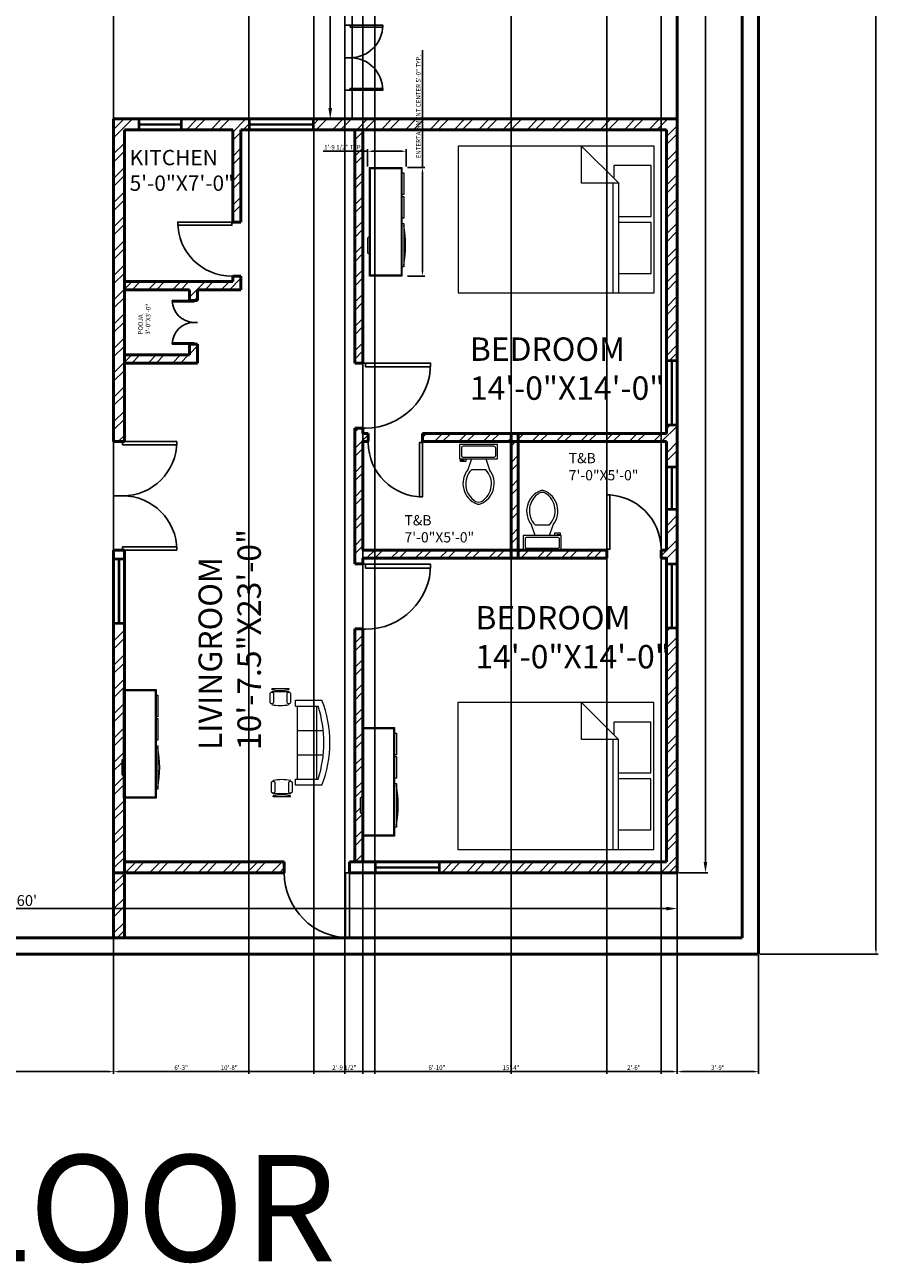
# Model space of a CAD drawing. Units: inches. Extents: x -12550 to 6516, y 1273 to 18700.
# Tile 3 of 19: x 2377 to 2849, y 1273 to 1958. Entities that reach past the tile are written whole.
import ezdxf

# ---------------------------------------------------------------- set-up
doc = ezdxf.new("R2010")
doc.units = ezdxf.units.IN
for name, color, linetype, lineweight in [('A-ANNO-DIMS', 2, 'Continuous', 18), ('A-ANNO-TEXT', 7, 'Continuous', 25), ('A-AREA-IDEN', 1, 'Continuous', 18), ('A-DOOR', 5, 'Continuous', 25), ('A-EQPM', 4, 'Continuous', 25), ('A-FURN', 8, 'Continuous', 18), ('A-GLAZ', 3, 'Continuous', 25), ('A-WALL', 7, 'Continuous', 50), ('A-WALL-PATT', 8, 'Continuous', 13)]:
    doc.layers.add(name, color=color, linetype=linetype, lineweight=lineweight)
doc.styles.get("Standard").update_dxf_attribs({"font": 'arial.ttf'})
doc.dimstyles.new('ISO-25', dxfattribs={"dimtxt": 2.5, "dimasz": 2.5, "dimexe": 1.25, "dimexo": 0.625, "dimtad": 1, "dimlunit": 4, "dimtxsty": 'Standard', "dimcen": 2.5, "dimadec": 0, "dimazin": 0, "dimtfac": 1, "dimtmove": 0, "dimatfit": 3, "dimfxl": 1, "dimarcsym": 0})

# ---------------------------------------------------------------- blocks, each defined once
blk = doc.blocks.new('*U2')
for p, q in [((0, 0), (0, -5)), ((30, 0), (30, -5))]:
    blk.add_line(p, q)
blk.add_lwpolyline([(0, 0), (0, 30), (1.75, 30), (1.75, 0)], close=True)
blk.add_arc((0, 0), 30, 0, 90)
blk = doc.blocks.new('Bed - Queen')
for p, q in [((0, -80.00003), (0, 0)), ((0, 0), (59.99999, 0)), ((59.99999, 0), (59.99999, -80.00003)), ((7.99999, -1.2), (28.79998, -1.2)), ((7.99999, -14.4), (7.99999, -1.2)), ((28.79998, -1.2), (28.79998, -14.4)), ((31.19999, -1.2), (51.99999, -1.2)), ((31.19999, -14.4), (31.19999, -1.2)), ((51.99999, -1.2), (51.99999, -16.4)), ((0, -14.4), (44.8, -14.4)), ((59.99999, -29.6), (44.8, -14.4)), ((44.8, -14.4), (44.8, -29.6)), ((44.8, -16.8), (0, -16.8)), ((51.99999, -16.4), (46.79936, -16.4)), ((44.8, -29.6), (59.99999, -29.6)), ((59.99999, -80.00003), (0, -80.00003))]:
    blk.add_line(p, q)
blk = doc.blocks.new('Toilet - top')
for p, q in [((9.5, -6), (9.5, -2)), ((-10, -8.5), (-8, -8.5)), ((-10, -9.5), (-10, -8.5)), ((-7, -9.5), (-10, -9.5)), ((-8, -8.5), (-8, -8)), ((-7, -8), (-7, -9.5)), ((-4, -8), (-6, -14)), ((4, -8), (6, -14)), ((4, -14), (-4, -14))]:
    blk.add_line(p, q)
blk.add_lwpolyline([(10.5, -8), (10.5, 0), (-10.5, 0), (-10.5, -8)], close=True)
for points in [[(-9.5, -2), (-9.5, -6)], [(8.5, -1), (-8.5, -1)], [(-8.5, -7), (8.5, -7)]]:
    blk.add_lwpolyline(points)
for centre, radius, start, end in [((-8.62, -1.88), 0.884, 81.8699, 188.1301), ((-8.62, -6.12), 0.884, 171.8699, 278.1301), ((8.62, -1.88), 0.884, 351.8699, 98.1301), ((8.62, -6.12), 0.884, 261.8699, 8.1301), ((3.52, -21.58), 12.17, 141.46911, 247.97143), ((4.2, -21.82), 11.33, 136.36773, 238.94682), ((-3.52, -21.58), 12.17, 292.02843, 38.53071), ((-4.2, -21.82), 11.33, 301.05301, 43.63209), ((0, -27.88), 4, 245.73182, 294.26817), ((0, -29), 4, 254.86053, 285.13947)]:
    blk.add_arc(centre, radius, start, end)
blk = doc.blocks.new('Entertainment Center')
for p, q in [((-4, 0), (-5, -1)), ((4, 0), (-4, 0)), ((5, -1), (4, 0)), ((-17, -19), (-17, -1)), ((-17, -1), (43, -1)), ((-16.5, -18.5), (-16.5, -1.5)), ((-16.5, -1.5), (42.5, -1.5)), ((42.5, -1.5), (42.5, -18.5)), ((43, -1), (43, -19)), ((43, -19), (-17, -19)), ((42.5, -18.5), (-16.5, -18.5)), ((-12, -20), (-12, -19)), ((12, -20), (-12, -20)), ((12, -19), (12, -20)), ((15, -20), (15, -19)), ((27, -20), (15, -20)), ((27, -19), (27, -20)), ((28, -20), (28, -19)), ((40, -20), (28, -20)), ((40, -19), (40, -20))]:
    blk.add_line(p, q)
blk.add_arc((0, 40), 61, 259.6111, 280.3889)
blk = doc.blocks.new('Sofa - Roundback 7 ft.')
for p, q in [((-36.000027, -34), (-36.000027, -11.4696)), ((-12.00002, -32.4421), (-12.00003, -6.5971)), ((11.99997, -32.4421), (11.99998, -6.5971)), ((35.99998, -34), (35.99998, -11.4696)), ((-35.999844, -13.3819), (35.9998, -13.3819)), ((-36.000027, -32.4421), (35.99998, -32.4421))]:
    blk.add_line(p, q)
for points in [[(-36.000027, -34), (-42.000027, -34), (-42.000027, -8)], [(41.99998, -8), (41.99998, -34), (35.99998, -34)]]:
    blk.add_lwpolyline(points)
for centre, radius, start, end in [((0, -114.25), 114.25, 68.43141, 111.5686), ((-0.00001, -127.1968), 121.1968, 72.72033, 107.2797)]:
    blk.add_arc(centre, radius, start, end)
blk = doc.blocks.new('Chair - Desk')
for p, q in [((-8.5, 0), (-8.5, -1)), ((-8.5, 0), (8.5, 0)), ((8.5, 0), (8.5, -1)), ((-10.5, -5), (-10.5, -14)), ((-8.5, -3), (-8.5, -4)), ((-8.5, -3), (8.5, -3)), ((-6.5, -14), (-6.5, -5)), ((-2, -3), (-2, -1.9355)), ((2, -1.9576), (2, -3)), ((6.5, -5), (6.5, -14)), ((8.5, -3), (8.5, -4)), ((10.5, -14), (10.5, -5)), ((-8.5, -15), (-8.5, -16)), ((8.5, -15), (8.5, -16))]:
    blk.add_line(p, q)
for centre, radius, start, end in [((-8.5, -6.5), 2.5, 36.8699, 143.1301), ((0, 34.625), 36.625, 256.5803, 283.4197), ((8.5, -6.5), 2.5, 36.8699, 143.1301), ((-8.5, -12.5), 2.5, 216.8699, 323.1301), ((0, 19.625), 36.625, 256.5803, 283.4197), ((8.5, -12.5), 2.5, 216.8699, 323.1301)]:
    blk.add_arc(centre, radius, start, end)
blk = doc.blocks.new('*D14')
at = {"layer": 'A-ANNO-DIMS', "color": 0, "lineweight": -2, "transparency": 16777216}
for p, q in [((2553.06, 2056.25), (2544.35, 2056.25)), ((2545.6, 2050.25), (2545.6, 1912.25)), ((2553.06, 1906.25), (2544.35, 1906.25))]:
    blk.add_line(p, q, dxfattribs=at)
at = {"layer": 'A-ANNO-DIMS', "color": 0, "transparency": 16777216}
for points in [[(2544.6, 2050.25), (2546.6, 2050.25), (2545.6, 2056.25)], [(2544.6, 1912.25), (2546.6, 1912.25), (2545.6, 1906.25)]]:
    blk.add_solid(points, dxfattribs=at)
at = {"layer": 'Defpoints', "color": 0, "transparency": 16777216}
for p in [(2553.69, 2056.25), (2545.6, 1906.25), (2553.69, 1906.25)]:
    blk.add_point(p, dxfattribs=at)
at = {"layer": 'A-ANNO-DIMS', "color": 0, "transparency": 16777216, "insert": (2541.91, 1981.25), "char_height": 6, "attachment_point": 5, "rotation": 90}
blk.add_mtext('12\'-6"', dxfattribs=at)
blk = doc.blocks.new('*D16')
at = {"layer": 'A-ANNO-DIMS', "color": 0, "lineweight": -2, "transparency": 16777216}
for p, q in [((2738.31, 2473.25), (2754.56, 2473.25)), ((2753.31, 2467.25), (2753.31, 1495.25)), ((2738.31, 1489.25), (2754.56, 1489.25))]:
    blk.add_line(p, q, dxfattribs=at)
at = {"layer": 'A-ANNO-DIMS', "color": 0, "transparency": 16777216}
for points in [[(2752.31, 2467.25), (2754.31, 2467.25), (2753.31, 2473.25)], [(2752.31, 1495.25), (2754.31, 1495.25), (2753.31, 1489.25)]]:
    blk.add_solid(points, dxfattribs=at)
at = {"layer": 'Defpoints', "color": 0, "transparency": 16777216}
for p in [(2737.69, 2473.25), (2737.69, 1489.25), (2753.31, 1489.25)]:
    blk.add_point(p, dxfattribs=at)
at = {"layer": 'A-ANNO-DIMS', "color": 0, "transparency": 16777216, "insert": (2749.62, 1981.25), "char_height": 6, "attachment_point": 5, "rotation": 90}
blk.add_mtext("82'", dxfattribs=at)
blk = doc.blocks.new('*D17')
at = {"layer": 'A-ANNO-DIMS', "color": 0, "lineweight": -2, "transparency": 16777216}
for p, q in [((2017.69, 1488.62), (2017.69, 1468.21)), ((2737.69, 1488.62), (2737.69, 1468.21)), ((2731.69, 1469.46), (2023.69, 1469.46))]:
    blk.add_line(p, q, dxfattribs=at)
at = {"layer": 'A-ANNO-DIMS', "color": 0, "transparency": 16777216}
for points in [[(2023.69, 1470.46), (2023.69, 1468.46), (2017.69, 1469.46)], [(2731.69, 1470.46), (2731.69, 1468.46), (2737.69, 1469.46)]]:
    blk.add_solid(points, dxfattribs=at)
at = {"layer": 'Defpoints', "color": 0, "transparency": 16777216}
for p in [(2017.69, 1489.25), (2737.69, 1489.25), (2017.69, 1469.46)]:
    blk.add_point(p, dxfattribs=at)
at = {"layer": 'A-ANNO-DIMS', "color": 0, "transparency": 16777216, "insert": (2377.69, 1473.15), "char_height": 6, "attachment_point": 5}
blk.add_mtext("60'", dxfattribs=at)
blk = doc.blocks.new('WIN-3FT')
for p, q in [((0, 0), (0, 6)), ((0, 6), (36.02, 6)), ((36.02, 0), (0, 0)), ((0.5, 0), (0.5, 6)), ((35.52, 3.2), (0.5, 3.2)), ((35.52, 2.8), (0.5, 2.8)), ((35.52, 6), (35.52, 0)), ((36.02, 6), (36.02, 0))]:
    blk.add_line(p, q)
blk = doc.blocks.new('WIN-2FT')
for p, q in [((0, 0), (0, 24.02)), ((0, 24.02), (6, 24.02)), ((0, 23.52), (6, 23.52)), ((2.8, 0.5), (2.8, 23.52)), ((3.2, 0.5), (3.2, 23.52)), ((6, 24.02), (6, 0)), ((6, 0.5), (0, 0.5)), ((6, 0), (0, 0))]:
    blk.add_line(p, q)
blk = doc.blocks.new('*D67')
at = {"layer": 'A-ANNO-DIMS', "color": 0, "lineweight": -2, "transparency": 16777216}
for p, q in [((2596.65, 1879.38), (2596.65, 1944.22)), ((2588.28, 1879.38), (2597.9, 1879.38)), ((2596.65, 1821.88), (2596.65, 1876.88)), ((2588.28, 1819.38), (2597.9, 1819.38))]:
    blk.add_line(p, q, dxfattribs=at)
at = {"layer": 'A-ANNO-DIMS', "color": 0, "transparency": 16777216}
for points in [[(2596.24, 1876.88), (2597.07, 1876.88), (2596.65, 1879.38)], [(2596.24, 1821.88), (2597.07, 1821.88), (2596.65, 1819.38)]]:
    blk.add_solid(points, dxfattribs=at)
at = {"layer": 'Defpoints', "color": 0, "transparency": 16777216}
for p in [(2587.65, 1879.38), (2596.65, 1879.38), (2587.65, 1819.38)]:
    blk.add_point(p, dxfattribs=at)
at = {"layer": 'A-ANNO-DIMS', "color": 0, "transparency": 16777216, "insert": (2594.73, 1913.05), "char_height": 2.5, "attachment_point": 5, "rotation": 90}
blk.add_mtext('ENTERTAINMENT CENTER 5\'-0" TYP.', dxfattribs=at)
blk = doc.blocks.new('*D68')
at = {"layer": 'A-ANNO-DIMS', "color": 0, "lineweight": -2, "transparency": 16777216}
for p, q in [((2566.32, 1888.38), (2541.74, 1888.38)), ((2566.32, 1880), (2566.32, 1889.63)), ((2585.15, 1888.38), (2568.82, 1888.38)), ((2587.65, 1880), (2587.65, 1889.63))]:
    blk.add_line(p, q, dxfattribs=at)
at = {"layer": 'A-ANNO-DIMS', "color": 0, "transparency": 16777216}
for points in [[(2568.82, 1888.8), (2568.82, 1887.96), (2566.32, 1888.38)], [(2585.15, 1888.8), (2585.15, 1887.96), (2587.65, 1888.38)]]:
    blk.add_solid(points, dxfattribs=at)
at = {"layer": 'Defpoints', "color": 0, "transparency": 16777216}
for p in [(2566.32, 1888.38), (2566.32, 1879.38), (2587.65, 1879.38)]:
    blk.add_point(p, dxfattribs=at)
at = {"layer": 'A-ANNO-DIMS', "color": 0, "transparency": 16777216, "insert": (2552.78, 1890.3), "char_height": 2.5, "attachment_point": 5}
blk.add_mtext('1\'-9 1/2" TYP.', dxfattribs=at)
blk = doc.blocks.new('*D95')
at = {"layer": 'A-ANNO-DIMS', "color": 0, "lineweight": -2, "transparency": 16777216}
for p, q in [((2783.31, 2518.25), (2848.94, 2518.25)), ((2847.69, 1446.75), (2847.69, 2515.75)), ((2783.31, 1444.25), (2848.94, 1444.25))]:
    blk.add_line(p, q, dxfattribs=at)
at = {"layer": 'A-ANNO-DIMS', "color": 0, "transparency": 16777216}
for points in [[(2847.27, 2515.75), (2848.11, 2515.75), (2847.69, 2518.25)], [(2847.27, 1446.75), (2848.11, 1446.75), (2847.69, 1444.25)]]:
    blk.add_solid(points, dxfattribs=at)
at = {"layer": 'Defpoints', "color": 0, "transparency": 16777216}
for p in [(2782.69, 2518.25), (2847.69, 2518.25), (2782.69, 1444.25)]:
    blk.add_point(p, dxfattribs=at)
at = {"layer": 'A-ANNO-DIMS', "color": 0, "transparency": 16777216, "insert": (2845.79, 1981.25), "char_height": 2.5, "attachment_point": 5, "rotation": 90}
blk.add_mtext('89\'-6"', dxfattribs=at)
blk = doc.blocks.new('*D97')
at = {"layer": 'A-ANNO-DIMS', "color": 0, "lineweight": -2, "transparency": 16777216}
for p, q in [((2017.69, 1488.62), (2017.69, 1378)), ((2425.69, 1488.62), (2425.69, 1378)), ((2020.19, 1379.25), (2423.19, 1379.25))]:
    blk.add_line(p, q, dxfattribs=at)
at = {"layer": 'A-ANNO-DIMS', "color": 0, "transparency": 16777216}
for points in [[(2020.19, 1379.66), (2020.19, 1378.83), (2017.69, 1379.25)], [(2423.19, 1379.66), (2423.19, 1378.83), (2425.69, 1379.25)]]:
    blk.add_solid(points, dxfattribs=at)
at = {"layer": 'Defpoints', "color": 0, "transparency": 16777216}
for p in [(2017.69, 1489.25), (2425.69, 1489.25), (2425.69, 1379.25)]:
    blk.add_point(p, dxfattribs=at)
at = {"layer": 'A-ANNO-DIMS', "color": 0, "transparency": 16777216, "insert": (2221.69, 1381.15), "char_height": 2.5, "attachment_point": 5}
blk.add_mtext('34\'-0"', dxfattribs=at)
blk = doc.blocks.new('*D98')
at = {"layer": 'A-ANNO-DIMS', "color": 0, "lineweight": -2, "transparency": 16777216}
for p, q in [((2553.69, 1905.62), (2553.69, 1378)), ((2425.69, 1488.62), (2425.69, 1378)), ((2428.19, 1379.25), (2551.19, 1379.25))]:
    blk.add_line(p, q, dxfattribs=at)
at = {"layer": 'A-ANNO-DIMS', "color": 0, "transparency": 16777216}
for points in [[(2428.19, 1379.66), (2428.19, 1378.83), (2425.69, 1379.25)], [(2551.19, 1379.66), (2551.19, 1378.83), (2553.69, 1379.25)]]:
    blk.add_solid(points, dxfattribs=at)
at = {"layer": 'Defpoints', "color": 0, "transparency": 16777216}
for p in [(2553.69, 1906.25), (2425.69, 1489.25), (2553.69, 1379.25)]:
    blk.add_point(p, dxfattribs=at)
at = {"layer": 'A-ANNO-DIMS', "color": 0, "transparency": 16777216, "insert": (2489.69, 1381.15), "char_height": 2.5, "attachment_point": 5}
blk.add_mtext('10\'-8"', dxfattribs=at)
blk = doc.blocks.new('*D99')
at = {"layer": 'A-ANNO-DIMS', "color": 0, "lineweight": -2, "transparency": 16777216}
for p, q in [((2553.69, 1905.62), (2553.69, 1378)), ((2737.69, 1905.62), (2737.69, 1378)), ((2556.19, 1379.25), (2735.19, 1379.25))]:
    blk.add_line(p, q, dxfattribs=at)
at = {"layer": 'A-ANNO-DIMS', "color": 0, "transparency": 16777216}
for points in [[(2556.19, 1379.66), (2556.19, 1378.83), (2553.69, 1379.25)], [(2735.19, 1379.66), (2735.19, 1378.83), (2737.69, 1379.25)]]:
    blk.add_solid(points, dxfattribs=at)
at = {"layer": 'Defpoints', "color": 0, "transparency": 16777216}
for p in [(2553.69, 1906.25), (2737.69, 1906.25), (2737.69, 1379.25)]:
    blk.add_point(p, dxfattribs=at)
at = {"layer": 'A-ANNO-DIMS', "color": 0, "transparency": 16777216, "insert": (2645.69, 1381.15), "char_height": 2.5, "attachment_point": 5}
blk.add_mtext('15\'-4"', dxfattribs=at)
blk = doc.blocks.new('*D100')
at = {"layer": 'A-ANNO-DIMS', "color": 0, "lineweight": -2, "transparency": 16777216}
for p, q in [((2737.69, 1488.62), (2737.69, 1378)), ((2782.69, 1443.62), (2782.69, 1378)), ((2740.19, 1379.25), (2780.19, 1379.25))]:
    blk.add_line(p, q, dxfattribs=at)
at = {"layer": 'A-ANNO-DIMS', "color": 0, "transparency": 16777216}
for points in [[(2740.19, 1379.66), (2740.19, 1378.83), (2737.69, 1379.25)], [(2780.19, 1379.66), (2780.19, 1378.83), (2782.69, 1379.25)]]:
    blk.add_solid(points, dxfattribs=at)
at = {"layer": 'Defpoints', "color": 0, "transparency": 16777216}
for p in [(2737.69, 1489.25), (2782.69, 1444.25), (2782.69, 1379.25)]:
    blk.add_point(p, dxfattribs=at)
at = {"layer": 'A-ANNO-DIMS', "color": 0, "transparency": 16777216, "insert": (2760.19, 1381.15), "char_height": 2.5, "attachment_point": 5}
blk.add_mtext('3\'-9"', dxfattribs=at)
blk = doc.blocks.new('*D152')
at = {"layer": 'A-ANNO-DIMS', "color": 0, "lineweight": -2, "transparency": 16777216}
for p, q in [((2425.69, 2055.62), (2425.69, 1378)), ((2500.53, 2055.62), (2500.53, 1378)), ((2428.19, 1379.25), (2498.03, 1379.25))]:
    blk.add_line(p, q, dxfattribs=at)
at = {"layer": 'A-ANNO-DIMS', "color": 0, "transparency": 16777216}
for points in [[(2428.19, 1379.66), (2428.19, 1378.83), (2425.69, 1379.25)], [(2498.03, 1379.66), (2498.03, 1378.83), (2500.53, 1379.25)]]:
    blk.add_solid(points, dxfattribs=at)
at = {"layer": 'Defpoints', "color": 0, "transparency": 16777216}
for p in [(2425.69, 2056.25), (2500.53, 2056.25), (2500.53, 1379.25)]:
    blk.add_point(p, dxfattribs=at)
at = {"layer": 'A-ANNO-DIMS', "color": 0, "transparency": 16777216, "insert": (2463.11, 1381.15), "char_height": 2.5, "attachment_point": 5}
blk.add_mtext('6\'-3"', dxfattribs=at)
blk = doc.blocks.new('*D153')
at = {"layer": 'A-ANNO-DIMS', "color": 0, "lineweight": -2, "transparency": 16777216}
for p, q in [((2536.54, 2055.62), (2536.54, 1378)), ((2570.26, 2055.62), (2570.26, 1378)), ((2539.04, 1379.25), (2567.76, 1379.25))]:
    blk.add_line(p, q, dxfattribs=at)
at = {"layer": 'A-ANNO-DIMS', "color": 0, "transparency": 16777216}
for points in [[(2539.04, 1379.66), (2539.04, 1378.83), (2536.54, 1379.25)], [(2567.76, 1379.66), (2567.76, 1378.83), (2570.26, 1379.25)]]:
    blk.add_solid(points, dxfattribs=at)
at = {"layer": 'Defpoints', "color": 0, "transparency": 16777216}
for p in [(2536.54, 2056.25), (2570.26, 2056.25), (2570.26, 1379.25)]:
    blk.add_point(p, dxfattribs=at)
at = {"layer": 'A-ANNO-DIMS', "color": 0, "transparency": 16777216, "insert": (2553.4, 1381.16), "char_height": 2.5, "attachment_point": 5}
blk.add_mtext('2\'-9 1/2"', dxfattribs=at)
blk = doc.blocks.new('*D162')
at = {"layer": 'A-ANNO-DIMS', "color": 0, "lineweight": -2, "transparency": 16777216}
for p, q in [((2698.69, 2234.12), (2698.69, 1378)), ((2728.69, 2234.12), (2728.69, 1378)), ((2701.19, 1379.25), (2726.19, 1379.25))]:
    blk.add_line(p, q, dxfattribs=at)
at = {"layer": 'A-ANNO-DIMS', "color": 0, "transparency": 16777216}
for points in [[(2701.19, 1379.66), (2701.19, 1378.83), (2698.69, 1379.25)], [(2726.19, 1379.66), (2726.19, 1378.83), (2728.69, 1379.25)]]:
    blk.add_solid(points, dxfattribs=at)
at = {"layer": 'Defpoints', "color": 0, "transparency": 16777216}
for p in [(2698.69, 2234.75), (2728.69, 2234.75), (2728.69, 1379.25)]:
    blk.add_point(p, dxfattribs=at)
at = {"layer": 'A-ANNO-DIMS', "color": 0, "transparency": 16777216, "insert": (2713.69, 1381.15), "char_height": 2.5, "attachment_point": 5}
blk.add_mtext('2\'-6"', dxfattribs=at)
blk = doc.blocks.new('*D163')
at = {"layer": 'A-ANNO-DIMS', "color": 0, "lineweight": -2, "transparency": 16777216}
for p, q in [((2563.69, 2234.12), (2563.69, 1378)), ((2645.69, 2229.62), (2645.69, 1378)), ((2566.19, 1379.25), (2643.19, 1379.25))]:
    blk.add_line(p, q, dxfattribs=at)
at = {"layer": 'A-ANNO-DIMS', "color": 0, "transparency": 16777216}
for points in [[(2566.19, 1379.66), (2566.19, 1378.83), (2563.69, 1379.25)], [(2643.19, 1379.66), (2643.19, 1378.83), (2645.69, 1379.25)]]:
    blk.add_solid(points, dxfattribs=at)
at = {"layer": 'Defpoints', "color": 0, "transparency": 16777216}
for p in [(2563.69, 2234.75), (2645.69, 2230.25), (2645.69, 1379.25)]:
    blk.add_point(p, dxfattribs=at)
at = {"layer": 'A-ANNO-DIMS', "color": 0, "transparency": 16777216, "insert": (2604.69, 1381.15), "char_height": 2.5, "attachment_point": 5}
blk.add_mtext('6\'-10"', dxfattribs=at)

msp = doc.modelspace()

# ---------------------------------------------------------------- hatches: boundary and pattern name
at = {"layer": 'A-WALL-PATT'}
h = msp.add_hatch(dxfattribs=at)
h.set_pattern_fill('ANSI32', color=256)
h.paths.add_polyline_path([(2439.446, 1906.247), (2425.689, 1906.247), (2425.689, 1727.747), (2430.689, 1727.747), (2431.689, 1727.747), (2431.689, 1900.247), (2439.446, 1900.247)])
h = msp.add_hatch(dxfattribs=at)
h.set_pattern_fill('ANSI32', color=256)
h.paths.add_polyline_path([(2500.528, 1906.247), (2463.463, 1906.247), (2463.463, 1900.247), (2491.689, 1900.247), (2491.689, 1849.247), (2496.189, 1849.247), (2496.189, 1900.247), (2500.528, 1900.247)])
h = msp.add_hatch(dxfattribs=at)
h.set_pattern_fill('ANSI32', color=256)
h.paths.add_polyline_path([(2737.689, 1906.247), (2559.189, 1906.247), (2536.545, 1906.247), (2536.545, 1900.247), (2559.189, 1900.247), (2731.689, 1900.247), (2731.689, 1772.747), (2737.689, 1772.747)])
h = msp.add_hatch(dxfattribs=at)
h.set_pattern_fill('ANSI32', color=256)
h.paths.add_polyline_path([(2563.689, 1900.247), (2559.189, 1900.247), (2559.189, 1771.247), (2563.689, 1771.247)])
h = msp.add_hatch(dxfattribs=at)
h.set_pattern_fill('ANSI32', color=256)
h.paths.add_polyline_path([(2496.189, 1819.247), (2491.689, 1819.247), (2491.689, 1816.247), (2431.689, 1816.247), (2431.689, 1811.747), (2467.689, 1811.747), (2467.689, 1805.747), (2470.189, 1805.747), (2472.189, 1805.747), (2472.189, 1811.747), (2496.189, 1811.747)])
h = msp.add_hatch(dxfattribs=at)
h.set_pattern_fill('ANSI32', color=256)
h.paths.add_polyline_path([(2472.189, 1781.747), (2470.189, 1781.747), (2467.689, 1781.747), (2467.689, 1775.747), (2431.689, 1775.747), (2431.689, 1771.247), (2472.189, 1771.247)])
h = msp.add_hatch(dxfattribs=at)
h.set_pattern_fill('ANSI32', color=256)
h.paths.add_polyline_path([(2563.689, 1727.747), (2566.689, 1727.747), (2566.689, 1732.247), (2563.689, 1732.247), (2563.689, 1735.247), (2559.189, 1735.247), (2559.189, 1660.247), (2563.689, 1660.247), (2563.689, 1663.247), (2566.641, 1663.247), (2645.689, 1663.247), (2645.689, 1667.747), (2566.641, 1667.747), (2563.689, 1667.747)])
h = msp.add_hatch(dxfattribs=at)
h.set_pattern_fill('ANSI32', color=256)
h.paths.add_polyline_path([(2737.689, 1736.73), (2731.689, 1736.73), (2731.689, 1732.247), (2728.689, 1732.247), (2649.689, 1732.247), (2649.689, 1727.747), (2728.689, 1727.747), (2731.689, 1727.747), (2731.689, 1714.042), (2737.689, 1714.042)])
h = msp.add_hatch(dxfattribs=at)
h.set_pattern_fill('ANSI32', color=256)
h.paths.add_polyline_path([(2645.689, 1732.247), (2596.689, 1732.247), (2596.689, 1727.747), (2645.689, 1727.747)], flags=17)
h = msp.add_hatch(dxfattribs=at)
h.set_pattern_fill('ANSI32', color=256)
h.paths.add_polyline_path([(2649.689, 1727.747), (2645.689, 1727.747), (2645.689, 1667.747), (2649.689, 1667.747)])
h = msp.add_hatch(dxfattribs=at)
h.set_pattern_fill('ANSI32', color=256)
h.paths.add_polyline_path([(2737.689, 1690.024), (2731.689, 1690.024), (2731.689, 1667.747), (2728.689, 1667.747), (2728.689, 1663.247), (2731.689, 1663.247), (2731.689, 1660.369), (2737.689, 1660.369)])
h = msp.add_hatch(dxfattribs=at)
h.set_pattern_fill('ANSI32', color=256)
h.paths.add_polyline_path([(2698.689, 1667.747), (2649.689, 1667.747), (2649.689, 1663.247), (2698.689, 1663.247)])
h = msp.add_hatch(dxfattribs=at)
h.set_pattern_fill('ANSI32', color=256)
h.paths.add_polyline_path([(2520.189, 1495.247), (2431.689, 1495.247), (2431.689, 1530.559), (2431.189, 1530.559), (2431.189, 1542.559), (2430.189, 1543.559), (2430.189, 1551.559), (2431.189, 1552.559), (2431.189, 1590.559), (2431.425, 1627.032), (2425.689, 1627.032), (2425.689, 1489.247), (2520.189, 1489.247)])
h = msp.add_hatch(dxfattribs=at)
h.set_pattern_fill('ANSI32', color=256)
h.paths.add_polyline_path([(2559.189, 1623.947), (2559.189, 1495.247), (2563.689, 1495.247), (2563.689, 1509.575), (2563.189, 1509.575), (2563.189, 1521.575), (2562.189, 1522.575), (2562.189, 1530.575), (2563.189, 1531.575), (2563.189, 1569.575), (2563.686, 1623.947)])
h = msp.add_hatch(dxfattribs=at)
h.set_pattern_fill('ANSI32', color=256)
h.paths.add_polyline_path([(2737.689, 1624.352), (2731.689, 1624.352), (2731.689, 1495.247), (2606.275, 1495.247), (2606.275, 1489.247), (2737.689, 1489.247)])
h = msp.add_hatch(dxfattribs=at)
h.set_pattern_fill('ANSI32', color=256)
h.paths.add_polyline_path([(2431.689, 1489.247), (2425.689, 1489.247), (2425.689, 1453.247), (2431.689, 1453.247)])

# ---------------------------------------------------------------- linework, layer by layer
at = {"layer": 'A-EQPM'}
for p, q in [((2553.689, 1906.247), (2553.689, 2056.247)), ((2557.689, 1906.247), (2557.689, 2056.247)), ((2737.689, 2056.247), (2737.689, 1906.247)), ((2737.689, 1906.247), (2553.689, 1906.247))]:
    msp.add_line(p, q, dxfattribs=at)
at = {"layer": 'A-WALL'}
for p, q in [((2782.689, 2518.247), (2782.689, 1444.247)), ((2773.689, 2509.247), (2773.689, 1453.247)), ((2737.689, 1489.247), (2737.689, 2060.923)), ((2773.689, 1489.247), (2773.689, 2060.923)), ((2559.189, 1906.247), (2425.689, 1906.247)), ((2425.689, 1727.747), (2425.689, 1906.247)), ((2737.689, 1906.247), (2559.189, 1906.247)), ((2431.689, 1727.747), (2431.689, 1900.247)), ((2491.689, 1900.247), (2431.689, 1900.247)), ((2491.689, 1849.247), (2491.689, 1900.247)), ((2559.189, 1900.247), (2496.189, 1900.247)), ((2496.189, 1849.247), (2496.189, 1900.247)), ((2731.689, 1900.247), (2559.189, 1900.247)), ((2559.189, 1771.247), (2559.189, 1900.247)), ((2563.689, 1771.247), (2563.689, 1900.247)), ((2731.689, 1732.247), (2731.689, 1900.247)), ((2491.689, 1849.247), (2496.189, 1849.247)), ((2491.689, 1816.247), (2431.689, 1816.247)), ((2491.689, 1816.247), (2491.689, 1819.247)), ((2496.189, 1819.247), (2491.689, 1819.247)), ((2496.189, 1811.747), (2496.189, 1819.247)), ((2496.189, 1816.247), (2496.189, 1819.247)), ((2467.689, 1811.747), (2431.689, 1811.747)), ((2467.689, 1805.747), (2467.689, 1811.747)), ((2496.189, 1811.747), (2472.189, 1811.747)), ((2472.189, 1805.747), (2472.189, 1811.747)), ((2467.689, 1805.747), (2472.189, 1805.747)), ((2467.689, 1775.747), (2467.689, 1781.747)), ((2472.189, 1781.747), (2467.689, 1781.747)), ((2472.189, 1771.247), (2472.189, 1781.747)), ((2472.189, 1775.747), (2472.189, 1781.747)), ((2467.689, 1775.747), (2431.689, 1775.747)), ((2472.189, 1771.247), (2431.689, 1771.247)), ((2559.189, 1771.247), (2563.689, 1771.247)), ((2563.689, 1735.247), (2559.189, 1735.247)), ((2559.189, 1660.247), (2559.189, 1735.247)), ((2563.689, 1732.247), (2563.689, 1735.247)), ((2563.689, 1732.247), (2563.689, 1735.247)), ((2563.689, 1732.247), (2563.689, 1735.247)), ((2563.689, 1732.247), (2563.689, 1735.247)), ((2431.689, 1727.747), (2425.689, 1727.747)), ((2566.689, 1732.247), (2563.689, 1732.247)), ((2563.689, 1667.747), (2563.689, 1727.747)), ((2563.689, 1667.747), (2563.689, 1727.747)), ((2563.689, 1667.747), (2563.689, 1727.747)), ((2563.689, 1727.747), (2566.689, 1727.747)), ((2566.689, 1727.747), (2563.689, 1727.747)), ((2566.689, 1727.747), (2566.689, 1732.247)), ((2728.689, 1732.247), (2596.689, 1732.247)), ((2596.689, 1732.247), (2596.689, 1727.747)), ((2728.689, 1727.747), (2596.689, 1727.747)), ((2645.689, 1663.247), (2645.689, 1732.247)), ((2649.689, 1663.247), (2649.689, 1732.247)), ((2731.689, 1732.247), (2728.689, 1732.247)), ((2731.689, 1732.247), (2728.689, 1732.247)), ((2731.689, 1727.747), (2728.689, 1727.747)), ((2731.689, 1667.747), (2731.689, 1727.747)), ((2431.689, 1667.747), (2425.689, 1667.747)), ((2425.689, 1453.247), (2425.689, 1667.747)), ((2431.689, 1453.247), (2431.689, 1667.747)), ((2566.641, 1667.747), (2563.689, 1667.747)), ((2698.689, 1667.747), (2566.641, 1667.747)), ((2698.689, 1667.747), (2698.689, 1663.247)), ((2731.689, 1667.747), (2728.689, 1667.747)), ((2728.689, 1663.247), (2728.689, 1667.747)), ((2559.189, 1663.247), (2559.189, 1660.247)), ((2559.189, 1660.247), (2563.689, 1660.247)), ((2563.689, 1660.247), (2563.689, 1663.247)), ((2563.689, 1660.247), (2563.689, 1663.247)), ((2563.689, 1660.247), (2563.689, 1663.247)), ((2566.641, 1663.247), (2563.689, 1663.247)), ((2698.689, 1663.247), (2566.641, 1663.247)), ((2731.689, 1663.247), (2728.689, 1663.247)), ((2731.689, 1663.247), (2728.689, 1663.247)), ((2731.689, 1495.247), (2731.689, 1663.247)), ((2559.189, 1495.247), (2559.189, 1624.247)), ((2563.689, 1624.247), (2559.189, 1624.247)), ((2563.689, 1495.247), (2563.689, 1624.247)), ((2520.189, 1495.247), (2431.689, 1495.247)), ((2520.189, 1489.247), (2520.189, 1495.247)), ((2731.689, 1495.247), (2556.189, 1495.247)), ((2559.189, 1495.247), (2556.189, 1495.247)), ((2556.189, 1495.247), (2556.189, 1489.247)), ((2520.189, 1489.247), (2425.689, 1489.247)), ((2737.689, 1489.247), (2556.189, 1489.247)), ((1981.689, 1453.247), (2773.689, 1453.247)), ((2520.189, 1453.247), (2256.189, 1453.247)), ((1972.689, 1444.247), (2782.689, 1444.247))]:
    msp.add_line(p, q, dxfattribs=at)

# ---------------------------------------------------------------- block references
at = {"layer": 'A-DOOR', "xscale": -1}
for p, rotation in [((2491.189, 1849.247), 90), ((2430.689, 1667.747), 270)]:
    msp.add_blockref('*U2', p, dxfattribs=dict(at, rotation=rotation))
at = {"layer": 'A-DOOR'}
for p, xscale, yscale, zscale, rotation in [((2470.189, 1805.747), -0.399999999999997, 0.399999999999997, 0.399999999999997, 90), ((2470.189, 1781.747), 0.399999999999997, 0.399999999999997, 0.399999999999997, 90.00000000000003), ((2565.189, 1771.247), 1.199999999999999, 1.199999999999999, 1.199999999999999, 270), ((2565.189, 1659.947), 1.199999999999999, 1.199999999999999, 1.199999999999999, 270), ((2556.189, 1489.247), 1.199999999999999, 1.199999999999999, 1.199999999999999, 180)]:
    msp.add_blockref('*U2', p, dxfattribs=dict(at, xscale=xscale, yscale=yscale, zscale=zscale, rotation=rotation))
for p, rotation in [((2430.689, 1727.747), 270), ((2596.689, 1727.247), 180)]:
    msp.add_blockref('*U2', p, dxfattribs=dict(at, rotation=rotation))
msp.add_blockref('*U2', (2698.689, 1668.247), dxfattribs=at)
at = {"layer": 'A-EQPM', "yscale": 0.5999999999999954, "zscale": 0.5999999999999954, "rotation": 270}
for p, xscale in [((2556.689, 1958.135), 0.5999999999999954), ((2556.689, 1922.135), -0.5999999999999954)]:
    msp.add_blockref('*U2', p, dxfattribs=dict(at, xscale=xscale))
at = {"layer": 'A-FURN'}
for name, p, xscale, yscale, zscale, rotation in [('Bed - Queen', (2724.868, 1809.994), -1.354827908062564, 1.354827908062564, 1.354827908062564, 270), ('Sofa - Roundback 7 ft.', (2545.408, 1561.265), 0.5595223685495907, 0.5595223685495907, 0.5595223685495907, 270), ('Bed - Queen', (2724.708, 1502.217), -1.354827908062564, 1.354827908062564, 1.354827908062564, 270), ('Chair - Desk', (2518.822, 1531.281), 0.5595223685495907, 0.5595223685495907, 0.5595223685495907, 180)]:
    msp.add_blockref(name, p, dxfattribs=dict(at, xscale=xscale, yscale=yscale, zscale=zscale, rotation=rotation))
for name, p, rotation in [('Entertainment Center', (2566.318, 1836.379), 89.99999999999999), ('Toilet - top', (2662.958, 1667.747), 180), ('Entertainment Center', (2430.189, 1547.559), 89.99999999999999), ('Entertainment Center', (2562.189, 1526.575), 89.99999999999999)]:
    msp.add_blockref(name, p, dxfattribs=dict(at, rotation=rotation))
msp.add_blockref('Toilet - top', (2627.711, 1726.198), dxfattribs=at)
at = {"layer": 'A-FURN', "xscale": 0.5595223685495907, "yscale": 0.5595223685495907, "zscale": 0.5595223685495907}
msp.add_blockref('Chair - Desk', (2517.969, 1591.265), dxfattribs=at)
at = {"layer": 'A-GLAZ'}
for name, p, rotation in [('WIN-2FT', (2439.446, 1906.247), 269.9999999999959), ('WIN-3FT', (2536.545, 1906.247), 180), ('WIN-3FT', (2737.689, 1736.73), 90.00000000000058), ('WIN-2FT', (2737.689, 1714.042), 180), ('WIN-3FT', (2431.689, 1627.032), 90.00000000000058), ('WIN-3FT', (2737.689, 1624.352), 90.00000000000047), ('WIN-3FT', (2606.275, 1495.247), 180)]:
    msp.add_blockref(name, p, dxfattribs=dict(at, rotation=rotation))

# ---------------------------------------------------------------- texts
at = {"layer": 'A-ANNO-TEXT', "insert": (2160.68, 1333.138), "char_height": 58.816, "attachment_point": 1}
msp.add_mtext('1st FLOOR', dxfattribs=at)
at = {"layer": 'A-AREA-IDEN', "attachment_point": 1}
for s, width, gutter_width, insert, char_height in [('KITCHEN\\P5\'-0"X7\'-0"', 1.29487, 42.422, (2434.569, 1889.124), 8.48435), ('T&B\\P7\'-0"X5\'-0"', 4.19569, 28.328, (2677.611, 1721.465), 5.66556), ('T&B\\P7\'-0"X5\'-0"', 4.19569, 28.328, (2586.701, 1687.107), 5.66556)]:
    msp.add_mtext_dynamic_manual_height_columns(s, width=width, gutter_width=gutter_width, heights=[0], dxfattribs=dict(at, insert=insert, char_height=char_height))
at = {"layer": 'A-AREA-IDEN', "insert": (2439.241, 1787.026), "char_height": 2.5, "attachment_point": 1, "rotation": 89.183853}
msp.add_mtext_dynamic_manual_height_columns('POOJA\\P3\'-0"X3\'-0"', width=0.78585, gutter_width=12.5, heights=[0], dxfattribs=at)
at = {"layer": 'A-AREA-IDEN', "char_height": 12.93169, "attachment_point": 1}
for insert in [(2622.904, 1785.378), (2625.969, 1636.812)]:
    msp.add_mtext('BEDROOM\\P14\'-0"X14\'-0"', dxfattribs=dict(at, insert=insert))
at = {"layer": 'A-AREA-IDEN', "insert": (2472.713, 1557.153), "char_height": 12.93169, "attachment_point": 1, "rotation": 90}
msp.add_mtext('LIVINGROOM\\P10\'-7.5"X23\'-0"', dxfattribs=at)

# ---------------------------------------------------------------- dimensions: what is measured, and where the dimension line sits
at = {"layer": 'A-ANNO-DIMS'}
for base, p1, p2, override, picture, middle in [((2847.689, 2518.247), (2782.689, 1444.247), (2782.689, 2518.247), {"dimdec": 1, "dimlfac": 1, "dimrnd": 0, "dimzin": 1, "dimdsep": 46, "dimlunit": 4, "dimfrac": 2}, '*D95', (2845.787, 1981.247)), ((2753.309, 1489.247), (2737.689, 2473.247), (2737.689, 1489.247), {"dimtxt": 6, "dimasz": 6, "dimclrd": 0, "dimclre": 0, "dimclrt": 0}, '*D16', (2749.62, 1981.247)), ((2545.602, 1906.247), (2553.689, 2056.247), (2553.689, 1906.247), {"dimtxt": 6, "dimasz": 6, "dimclrd": 0, "dimclre": 0, "dimclrt": 0}, '*D14', (2541.914, 1981.247))]:
    dim = msp.add_linear_dim(base=base, p1=p1, p2=p2, angle=90, dimstyle='ISO-25', override=override, dxfattribs=at)
    dim.commit()
    dim.dimension.update_dxf_attribs({"geometry": picture, "text_midpoint": middle})
for base, p1, p2, override, picture, middle in [((2645.689, 1379.247), (2563.689, 2234.747), (2645.689, 2230.247), {"dimdec": 1, "dimlfac": 1, "dimrnd": 0, "dimzin": 1, "dimdsep": 46, "dimlunit": 4, "dimfrac": 2}, '*D163', (2604.689, 1381.149)), ((2728.689, 1379.247), (2698.689, 2234.747), (2728.689, 2234.747), {"dimdec": 1, "dimlfac": 1, "dimrnd": 0, "dimzin": 1, "dimdsep": 46, "dimlunit": 4, "dimfrac": 2}, '*D162', (2713.689, 1381.149)), ((2500.528, 1379.247), (2425.689, 2056.247), (2500.528, 2056.247), {"dimdec": 1, "dimlfac": 1, "dimrnd": 0, "dimzin": 1, "dimdsep": 46, "dimlunit": 4, "dimfrac": 2}, '*D152', (2463.108, 1381.15)), ((2570.258, 1379.247), (2536.545, 2056.247), (2570.258, 2056.247), {"dimdec": 1, "dimlfac": 1, "dimrnd": 0, "dimzin": 1, "dimdsep": 46, "dimlunit": 4, "dimfrac": 2}, '*D153', (2553.401, 1381.165)), ((2553.689, 1379.247), (2425.689, 1489.247), (2553.689, 1906.247), {"dimdec": 1, "dimlfac": 1, "dimrnd": 0, "dimzin": 1, "dimdsep": 46, "dimlunit": 4, "dimfrac": 2}, '*D98', (2489.689, 1381.149)), ((2737.689, 1379.247), (2553.689, 1906.247), (2737.689, 1906.247), {"dimdec": 1, "dimlfac": 1, "dimrnd": 0, "dimzin": 1, "dimdsep": 46, "dimlunit": 4, "dimfrac": 2}, '*D99', (2645.689, 1381.149)), ((2017.689, 1469.461), (2737.689, 1489.247), (2017.689, 1489.247), {"dimtxt": 6, "dimasz": 6, "dimclrd": 0, "dimclre": 0, "dimclrt": 0}, '*D17', (2377.689, 1473.15)), ((2425.689, 1379.247), (2017.689, 1489.247), (2425.689, 1489.247), {"dimdec": 1, "dimlfac": 1, "dimrnd": 0, "dimzin": 1, "dimdsep": 46, "dimlunit": 4, "dimfrac": 2}, '*D97', (2221.689, 1381.15)), ((2782.689, 1379.247), (2737.689, 1489.247), (2782.689, 1444.247), {"dimdec": 1, "dimlfac": 1, "dimrnd": 0, "dimzin": 1, "dimdsep": 46, "dimlunit": 4, "dimfrac": 2}, '*D100', (2760.189, 1381.15))]:
    dim = msp.add_linear_dim(base=base, p1=p1, p2=p2, dimstyle='ISO-25', override=override, dxfattribs=at)
    dim.commit()
    dim.dimension.update_dxf_attribs({"geometry": picture, "text_midpoint": middle})
for base, p1, p2, angle, text, picture, middle in [((2596.652, 1879.379), (2587.652, 1819.379), (2587.652, 1879.379), 90, 'ENTERTAINMENT CENTER <> TYP.', '*D67', (2594.734, 1913.051)), ((2566.318, 1888.379), (2587.652, 1879.379), (2566.318, 1879.379), 180, '<> TYP.', '*D68', (2552.779, 1890.297))]:
    dim = msp.add_linear_dim(base=base, p1=p1, p2=p2, angle=angle, text=text, dimstyle='ISO-25', override={"dimdec": 1, "dimrnd": 0, "dimzin": 1, "dimlunit": 4, "dimfrac": 2}, dxfattribs=at)
    dim.commit()
    dim.dimension.update_dxf_attribs({"geometry": picture, "text_midpoint": middle})

doc.saveas('drawing.dxf')
